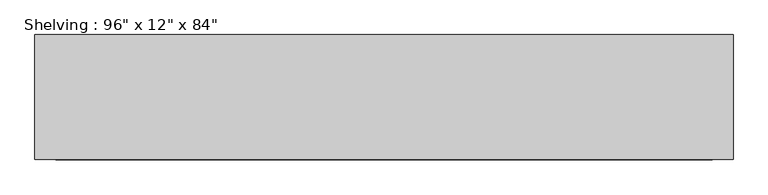
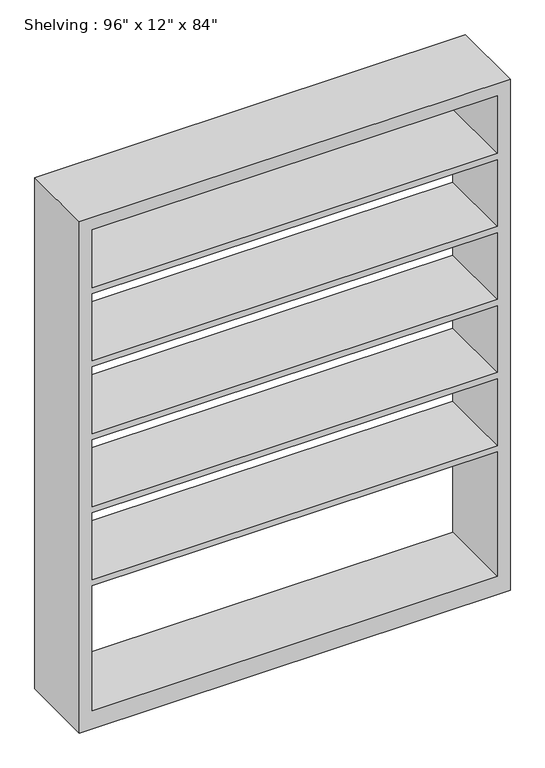
"""IFC4 building model written with IfcOpenShell, lengths in millimetres: furniture geometry."""

from ifc_helpers import new_model, si_unit, frame, origin, place, context, project, spatial, polyline, outline, extrude, source, transform, mapped, element, save


def furniture_fcf97a65(model_context):
    return source(origin(), model_context, "Body", "SweptSolid", [
        extrude(outline(polyline([(0.0, 850.9), (2133.6, 850.9), (2133.6, -850.9), (0.0, -850.9), (0.0, 850.9)]), holes=[polyline([(2082.8, 800.1), (1841.5, 800.1), (1841.5, -800.1), (2082.8, -800.1), (2082.8, 800.1)]), polyline([(76.2, 800.1), (76.2, -800.1), (596.9, -800.1), (596.9, 800.1), (76.2, 800.1)]), polyline([(1231.9, -800.1), (1511.3, -800.1), (1511.3, 800.1), (1231.9, 800.1), (1231.9, -800.1)]), polyline([(1816.1, 800.1), (1536.7, 800.1), (1536.7, -800.1), (1816.1, -800.1), (1816.1, 800.1)]), polyline([(1206.5, 800.1), (927.1, 800.1), (927.1, -800.1), (1206.5, -800.1), (1206.5, 800.1)]), polyline([(901.7, 800.1), (622.3, 800.1), (622.3, -800.1), (901.7, -800.1), (901.7, 800.1)])]), frame((0.0, -457.2, 0.0), z_axis=(0.0, 1.0, 0.0), x_axis=(0.0, 0.0, 1.0)), (0.0, 0.0, 1.0), 304.8),
    ])


if __name__ == "__main__":
    model = new_model("IFC4")
    model_context = context("Model", 3, world=origin())
    ifc_project = project(units=[si_unit("LENGTHUNIT", "METRE", prefix="MILLI")], contexts=[model_context])
    site = spatial("IfcSite", under=ifc_project)
    building = spatial("IfcBuilding", under=site)
    placement = place(None, origin())
    furniture_shape = furniture_fcf97a65(model_context)
    element("IfcFurniture", 1, ObjectType="Shelving : 96\" x 12\" x 84\"", at=placement, inside=building, context=model_context, shape_type="MappedRepresentation", body=[
        mapped(furniture_shape, transform((0.0, 0.0, 0.0), x_axis=(1.0, 0.0, 0.0), y_axis=(0.0, 1.0, 0.0), z_axis=(0.0, 0.0, 1.0))),
    ])
    save(model, "model.ifc")

# Revit data of these elements
# Type "Shelving : 96\" x 12\" x 84\""
#   Assembly Code = "E2020200"
#   Depth = 1' - 0"
#   Height = 7' - 0"
#   Width = 5' - 7"
#   Shelving Unit Material = Laminate, Ivory, Matte
#   Default Elevation = 0
# Element 1 (IfcFurniture, "Shelving : 96\" x 12\" x 84\"")
#   Materials on its faces: "Laminate, Ivory, Matte"
# Materials
#   "Laminate, Ivory, Matte": class "Plastic", colour RGB 247 247 239, transparency 0, Description = "Plastic Laminate - Ivory, Matte", Cost = 0
